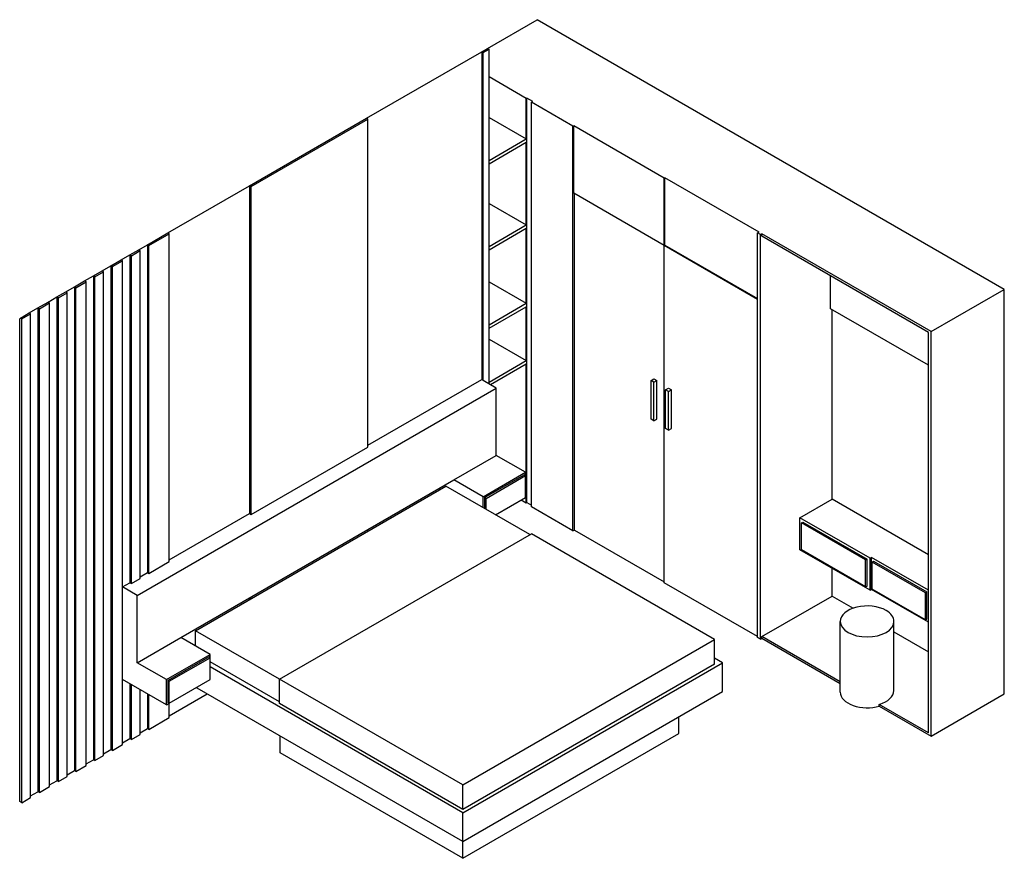
# Model space of a CAD drawing. Units: centimetres. Extents: x 2482 to 32323, y -172 to 5164.
# Tile 1 of 1: x 26482 to 32323, y 189 to 5164. Entities that reach past the tile are written whole.
import ezdxf

# ---------------------------------------------------------------- set-up
doc = ezdxf.new("R2010")
doc.units = ezdxf.units.CM
doc.header["$MEASUREMENT"] = 0
doc.layers.add('A-FURN', color=8, linetype='Continuous', lineweight=25)

msp = doc.modelspace()

# ---------------------------------------------------------------- linework, layer by layer
at = {"layer": 'A-FURN'}
for p, q in [((29257.4, 4994.3), (29551.8, 5164.3)), ((32323.1, 3564.3), (29551.8, 5164.3)), ((28538.6, 4579.3), (29222.7, 4974.3)), ((29222.7, 4974.3), (29257.4, 4994.3)), ((29231.4, 4969.3), (29222.7, 4974.3)), ((29222.7, 4974.3), (29222.7, 3029.3)), ((29231.4, 4969.3), (29266, 4989.3)), ((29231.4, 3024.3), (29231.4, 4969.3)), ((29257.4, 4994.3), (29266, 4989.3)), ((29266, 3004.3), (29266, 4989.3)), ((29486.9, 4696.8), (29266, 4824.3)), ((29486.9, 4696.8), (29491.2, 4699.3)), ((29486.9, 4456.8), (29486.9, 4696.8)), ((29525.8, 4679.3), (29491.2, 4699.3)), ((29491.2, 2299.3), (29491.2, 4699.3)), ((29517.2, 4674.3), (29525.8, 4679.3)), ((29764, 4531.8), (29517.2, 4674.3)), ((29517.2, 2274.3), (29517.2, 4674.3)), ((27845.7, 4179.3), (28538.6, 4579.3)), ((27854.4, 4174.3), (28547.2, 4574.3)), ((28547.2, 4574.3), (28538.6, 4579.3)), ((28547.2, 2629.3), (28547.2, 4574.3)), ((29266, 4584.3), (29486.9, 4456.8)), ((29764, 4531.8), (29768.3, 4534.3)), ((29764, 2131.8), (29764, 4531.8)), ((30305.3, 4224.3), (29768.3, 4534.3)), ((29768.3, 4134.3), (29768.3, 4534.3)), ((29266, 4329.3), (29486.9, 4456.8)), ((29266, 4309.3), (29486.9, 4436.8)), ((29486.9, 3946.8), (29486.9, 4436.8)), ((30305.3, 4224.3), (30309.6, 4226.8)), ((30305.3, 3824.3), (30305.3, 4224.3)), ((30868.2, 3904.3), (30309.6, 4226.8)), ((30309.6, 3826.8), (30309.6, 4226.8)), ((27360.8, 3899.3), (27845.7, 4179.3)), ((27845.7, 4179.3), (27845.7, 2234.3)), ((27854.4, 4174.3), (27845.7, 4179.3)), ((27854.4, 2229.3), (27854.4, 4174.3)), ((30305.3, 3824.3), (29768.3, 4134.3)), ((29772.7, 2136.8), (29772.7, 4131.8)), ((29266, 4074.3), (29486.9, 3946.8)), ((29266, 3819.3), (29486.9, 3946.8)), ((29266, 3799.3), (29486.9, 3926.8)), ((29486.9, 3481.8), (29486.9, 3926.8)), ((27239.5, 3829.3), (27360.8, 3899.3)), ((27248.2, 3824.3), (27369.4, 3894.3)), ((27369.4, 3894.3), (27360.8, 3899.3)), ((27369.4, 1949.3), (27369.4, 3894.3)), ((30859.5, 3899.3), (30868.2, 3904.3)), ((30876.8, 3889.3), (30859.5, 3899.3)), ((30859.5, 1499.3), (30859.5, 3899.3)), ((30876.8, 3889.3), (30885.5, 3894.3)), ((30876.8, 1489.3), (30876.8, 3889.3)), ((31890.1, 3314.3), (30885.5, 3894.3)), ((30885.5, 3879.3), (30885.5, 3894.3)), ((31872.8, 3309.3), (30885.5, 3879.3)), ((27135.6, 3769.3), (27187.6, 3799.3)), ((27187.6, 3799.3), (27239.5, 3829.3)), ((27196.2, 3794.3), (27187.6, 3799.3)), ((27239.5, 3829.3), (27239.5, 1884.3)), ((27248.2, 3824.3), (27239.5, 3829.3)), ((27248.2, 1879.3), (27248.2, 3824.3)), ((30305.3, 3824.3), (30309.6, 3826.8)), ((30305.3, 1824.3), (30305.3, 3824.3)), ((30859.5, 3504.3), (30305.3, 3824.3)), ((30309.6, 3826.8), (30859.5, 3509.3)), ((27023, 3704.3), (27083.6, 3739.3)), ((27083.6, 3739.3), (27135.6, 3769.3)), ((27092.3, 3734.3), (27083.6, 3739.3)), ((27135.6, 3769.3), (27135.6, 1824.3)), ((27144.3, 3764.3), (27135.6, 3769.3)), ((27144.3, 3764.3), (27196.2, 3794.3)), ((27144.3, 1819.3), (27144.3, 3764.3)), ((27196.2, 1849.3), (27196.2, 3794.3)), ((26971.1, 3674.3), (27023, 3704.3)), ((27023, 3704.3), (27023, 834.3)), ((27031.7, 3699.3), (27023, 3704.3)), ((27031.7, 3699.3), (27092.3, 3734.3)), ((27031.7, 829.3), (27031.7, 3699.3)), ((27092.3, 864.3), (27092.3, 3734.3)), ((26867.1, 3614.3), (26919.1, 3644.3)), ((26919.1, 3644.3), (26971.1, 3674.3)), ((26919.1, 3644.3), (26919.1, 774.3)), ((26927.8, 3639.3), (26919.1, 3644.3)), ((26927.8, 3639.3), (26979.7, 3669.3)), ((26927.8, 769.3), (26927.8, 3639.3)), ((26979.7, 3669.3), (26971.1, 3674.3)), ((26979.7, 799.3), (26979.7, 3669.3)), ((31292.5, 3449.3), (31292.5, 3644.3)), ((26754.6, 3549.3), (26806.5, 3579.3)), ((26806.5, 3579.3), (26867.1, 3614.3)), ((26806.5, 3579.3), (26806.5, 709.3)), ((26815.2, 3574.3), (26806.5, 3579.3)), ((26815.2, 3574.3), (26875.8, 3609.3)), ((26815.2, 704.3), (26815.2, 3574.3)), ((26875.8, 3609.3), (26867.1, 3614.3)), ((26875.8, 739.3), (26875.8, 3609.3)), ((29266, 3609.3), (29486.9, 3481.8)), ((31890.1, 3314.3), (32323.1, 3564.3)), ((32323.1, 1164.3), (32323.1, 3564.3)), ((26650.6, 3489.3), (26702.6, 3519.3)), ((26702.6, 3519.3), (26754.6, 3549.3)), ((26702.6, 3519.3), (26702.6, 649.3)), ((26711.3, 3514.3), (26702.6, 3519.3)), ((26711.3, 3514.3), (26763.2, 3544.3)), ((26711.3, 644.3), (26711.3, 3514.3)), ((26763.2, 3544.3), (26754.6, 3549.3)), ((26763.2, 674.3), (26763.2, 3544.3)), ((26538, 3424.3), (26590, 3454.3)), ((26590, 3454.3), (26650.6, 3489.3)), ((26590, 3454.3), (26590, 584.3)), ((26598.7, 3449.3), (26590, 3454.3)), ((26598.7, 3449.3), (26659.3, 3484.3)), ((26598.7, 579.3), (26598.7, 3449.3)), ((26659.3, 3484.3), (26650.6, 3489.3)), ((26659.3, 614.3), (26659.3, 3484.3)), ((29266, 3354.3), (29486.9, 3481.8)), ((29266, 3334.3), (29486.9, 3461.8)), ((29486.9, 3141.8), (29486.9, 3461.8)), ((31872.8, 3114.3), (31292.5, 3449.3)), ((26481.8, 3389.3), (26486.1, 3394.3)), ((26481.8, 526.8), (26481.8, 3389.3)), ((26486.1, 3394.3), (26538, 3424.3)), ((26494.7, 3389.3), (26486.1, 3394.3)), ((26494.7, 3389.3), (26546.7, 3419.3)), ((26494.7, 519.3), (26494.7, 3389.3)), ((26546.7, 3419.3), (26538, 3424.3)), ((26546.7, 549.3), (26546.7, 3419.3)), ((31301.2, 2319.3), (31301.2, 3444.3)), ((31872.8, 934.3), (31872.8, 3309.3)), ((31890.1, 914.3), (31890.1, 3314.3)), ((29266, 3269.3), (29486.9, 3141.8)), ((29266, 3014.3), (29486.9, 3141.8)), ((29274.7, 2999.3), (29486.9, 3121.8)), ((29486.9, 2296.8), (29486.9, 3121.8)), ((27178.9, 1749.3), (29309.3, 2979.3)), ((28547.2, 2639.3), (29222.7, 3029.3)), ((29231.4, 3024.3), (29222.7, 3029.3)), ((29309.3, 2979.3), (29231.4, 3024.3)), ((29309.3, 2579.3), (29309.3, 2979.3)), ((30227.3, 3024.3), (30244.6, 3034.3)), ((30227.3, 2794.3), (30227.3, 3024.3)), ((30244.6, 3014.3), (30227.3, 3024.3)), ((30244.6, 3034.3), (30262, 3024.3)), ((30244.6, 3014.3), (30262, 3024.3)), ((30244.6, 2784.3), (30244.6, 3014.3)), ((30262, 2794.3), (30262, 3024.3)), ((30313.9, 2969.3), (30331.2, 2979.3)), ((30331.2, 2979.3), (30348.6, 2969.3)), ((30313.9, 2739.3), (30313.9, 2969.3)), ((30331.2, 2959.3), (30313.9, 2969.3)), ((30331.2, 2959.3), (30348.6, 2969.3)), ((30331.2, 2729.3), (30331.2, 2959.3)), ((30348.6, 2739.3), (30348.6, 2969.3)), ((30244.6, 2784.3), (30227.3, 2794.3)), ((30244.6, 2784.3), (30262, 2794.3)), ((30331.2, 2729.3), (30313.9, 2739.3)), ((30331.2, 2729.3), (30348.6, 2739.3)), ((27854.4, 2229.3), (28547.2, 2629.3)), ((29058.2, 2434.3), (29309.3, 2579.3)), ((29482.5, 2479.3), (29309.3, 2579.3)), ((29231.4, 2334.3), (29482.5, 2479.3)), ((29240, 2329.3), (29473.9, 2464.3)), ((29248.7, 2324.3), (29482.5, 2459.3)), ((29482.5, 2459.3), (29473.9, 2464.3)), ((29482.5, 2459.3), (29482.5, 2479.3)), ((29482.5, 2329.3), (29482.5, 2459.3)), ((27438.7, 1499.3), (29058.2, 2434.3)), ((27525.3, 1539.3), (29010.6, 2396.8)), ((29508.5, 2109.3), (29010.6, 2396.8)), ((29231.4, 2334.3), (29058.2, 2434.3)), ((28971.6, 2384.3), (28971.6, 2374.3)), ((29231.4, 2269.3), (29231.4, 2334.3)), ((29240, 2329.3), (29240, 2264.3)), ((29248.7, 2324.3), (29240, 2329.3)), ((29248.7, 2259.3), (29248.7, 2324.3)), ((29305, 2226.8), (29482.5, 2329.3)), ((29486.9, 2296.8), (29456.6, 2314.3)), ((29486.9, 2296.8), (29491.2, 2299.3)), ((29491.2, 2299.3), (29517.2, 2284.3)), ((31110.7, 2209.3), (31301.2, 2319.3)), ((31872.8, 1989.3), (31301.2, 2319.3)), ((27369.4, 1959.3), (27845.7, 2234.3)), ((27845.7, 2234.3), (27854.4, 2229.3)), ((29764, 2131.8), (29517.2, 2274.3)), ((31110.7, 2019.3), (31110.7, 2209.3)), ((31526.4, 1969.3), (31110.7, 2209.3)), ((31119.3, 2179.3), (31128, 2184.3)), ((31119.3, 2019.3), (31119.3, 2179.3)), ((31500.4, 1959.3), (31119.3, 2179.3)), ((31128, 2184.3), (31509, 1964.3)), ((28023.3, 1251.8), (29517.2, 2114.3)), ((28547.2, 2129.3), (28547.2, 2139.3)), ((30604, 1486.8), (29517.2, 2114.3)), ((29764, 2131.8), (29772.7, 2136.8)), ((29772.7, 2136.8), (30305.3, 1829.3)), ((31526.4, 1779.3), (31110.7, 2019.3)), ((31500.4, 1799.3), (31119.3, 2019.3)), ((27248.2, 1879.3), (27369.4, 1949.3)), ((31500.4, 1959.3), (31509, 1964.3)), ((31500.4, 1799.3), (31500.4, 1959.3)), ((31509, 1804.3), (31509, 1964.3)), ((31526.4, 1969.3), (31535, 1974.3)), ((31526.4, 1779.3), (31526.4, 1969.3)), ((31872.8, 1779.3), (31535, 1974.3)), ((31535, 1784.3), (31535, 1974.3)), ((31539.3, 1946.8), (31548, 1951.8)), ((31539.3, 1786.8), (31539.3, 1946.8)), ((31855.4, 1764.3), (31539.3, 1946.8)), ((31548, 1951.8), (31864.1, 1769.3)), ((27196.2, 1859.3), (27239.5, 1884.3)), ((27239.5, 1884.3), (27248.2, 1879.3)), ((31301.2, 1744.3), (31301.2, 1909.3)), ((27092.3, 1799.3), (27135.6, 1824.3)), ((27135.6, 1824.3), (27144.3, 1819.3)), ((27144.3, 1819.3), (27196.2, 1849.3)), ((30859.5, 1504.3), (30305.3, 1824.3)), ((27178.9, 1749.3), (27092.3, 1799.3)), ((31500.4, 1799.3), (31509, 1804.3)), ((31526.4, 1779.3), (31535, 1784.3)), ((31872.8, 1589.3), (31535, 1784.3)), ((31855.4, 1604.3), (31539.3, 1786.8)), ((31855.4, 1764.3), (31864.1, 1769.3)), ((31855.4, 1604.3), (31855.4, 1764.3)), ((31864.1, 1609.3), (31864.1, 1769.3)), ((27178.9, 1349.3), (27178.9, 1749.3)), ((27845.7, 1734.3), (27845.7, 1724.3)), ((27854.4, 1729.3), (27854.4, 1739.3)), ((30885.5, 1504.3), (31301.2, 1744.3)), ((31301.2, 1744.3), (31425.5, 1672.5)), ((31349.8, 1174.3), (31349.8, 1594.3)), ((31668.3, 1184.3), (31668.3, 1594.3)), ((31855.4, 1604.3), (31864.1, 1609.3)), ((28023.3, 1251.8), (27525.3, 1539.3)), ((27525.3, 1449.3), (27525.3, 1539.3)), ((31668.3, 1532.3), (31872.8, 1414.3)), ((27178.9, 1349.3), (27438.7, 1499.3)), ((27611.9, 1399.3), (27438.7, 1499.3)), ((29110.1, 624.3), (30604, 1486.8)), ((30604, 1341.8), (30604, 1486.8)), ((30876.8, 1489.3), (30859.5, 1499.3)), ((30876.8, 1489.3), (30885.5, 1494.3)), ((30885.5, 1494.3), (30885.5, 1504.3)), ((31349.8, 1236.2), (30885.5, 1504.3)), ((30885.5, 1494.3), (31349.8, 1226.2)), ((27352.1, 1249.3), (27178.9, 1349.3)), ((27352.1, 1249.3), (27611.9, 1399.3)), ((27360.8, 1244.3), (27603.3, 1384.3)), ((27369.4, 1239.3), (27611.9, 1379.3)), ((27611.9, 1379.3), (27603.3, 1384.3)), ((27611.9, 1379.3), (27611.9, 1399.3)), ((27611.9, 1249.3), (27611.9, 1379.3)), ((28023.3, 1116.8), (27611.9, 1354.3)), ((29110.1, 459.3), (30651.7, 1349.3)), ((30651.7, 1349.3), (30604, 1376.8)), ((30651.7, 1179.3), (30651.7, 1349.3)), ((29110.1, 459.3), (27611.9, 1324.3)), ((30604, 1341.8), (29110.1, 479.3)), ((27352.1, 1099.3), (27092.3, 1249.3)), ((27352.1, 1099.3), (27352.1, 1249.3)), ((27360.8, 1244.3), (27360.8, 1114.3)), ((27369.4, 1239.3), (27360.8, 1244.3)), ((27369.4, 1109.3), (27611.9, 1249.3)), ((27369.4, 1109.3), (27369.4, 1239.3)), ((29110.1, 624.3), (28023.3, 1251.8)), ((28023.3, 1106.8), (28023.3, 1251.8)), ((27135.6, 1224.3), (27135.6, 899.3)), ((27144.3, 894.3), (27144.3, 1219.3)), ((27196.2, 924.3), (27196.2, 1189.3)), ((27534, 1199.3), (27534, 1204.3)), ((29110.1, 289.3), (27534, 1199.3)), ((29110.1, 289.3), (30651.7, 1179.3)), ((27239.5, 1164.3), (27239.5, 959.3)), ((27248.2, 954.3), (27248.2, 1159.3)), ((27369.4, 1109.3), (27360.8, 1114.3)), ((27369.4, 1034.3), (27594.6, 1164.3)), ((31890.1, 914.3), (32323.1, 1164.3)), ((27352.1, 1099.3), (27369.4, 1109.3)), ((27369.4, 1024.3), (27369.4, 1109.3)), ((29110.1, 479.3), (28023.3, 1106.8)), ((31872.8, 934.3), (31581.5, 1102.4)), ((31581.5, 1092.4), (31581.5, 1102.4)), ((31581.5, 1092.4), (31890.1, 914.3)), ((27248.2, 954.3), (27369.4, 1024.3)), ((30391.9, 929.3), (30391.9, 1029.3)), ((27196.2, 934.3), (27239.5, 959.3)), ((27248.2, 954.3), (27239.5, 959.3)), ((27092.3, 874.3), (27135.6, 899.3)), ((27144.3, 894.3), (27135.6, 899.3)), ((27144.3, 894.3), (27196.2, 924.3)), ((28027.6, 814.3), (28027.6, 914.3)), ((29110.1, 189.3), (30391.9, 929.3)), ((26979.7, 809.3), (27023, 834.3)), ((27031.7, 829.3), (27023, 834.3)), ((27031.7, 829.3), (27092.3, 864.3)), ((26875.8, 749.3), (26919.1, 774.3)), ((26927.8, 769.3), (26919.1, 774.3)), ((26927.8, 769.3), (26979.7, 799.3)), ((29110.1, 189.3), (28027.6, 814.3)), ((26763.2, 684.3), (26806.5, 709.3)), ((26815.2, 704.3), (26806.5, 709.3)), ((26815.2, 704.3), (26875.8, 739.3)), ((26659.3, 624.3), (26702.6, 649.3)), ((26711.3, 644.3), (26702.6, 649.3)), ((26711.3, 644.3), (26763.2, 674.3)), ((26546.7, 559.3), (26590, 584.3)), ((26598.7, 579.3), (26590, 584.3)), ((26598.7, 579.3), (26659.3, 614.3)), ((29110.1, 479.3), (29110.1, 624.3)), ((26494.7, 519.3), (26481.8, 526.8)), ((26494.7, 519.3), (26546.7, 549.3)), ((29110.1, 289.3), (29110.1, 459.3)), ((29110.1, 189.3), (29110.1, 289.3))]:
    msp.add_line(p, q, dxfattribs=at)
for centre, start_param, end_param in [((31509, 1594.3), 0.785398, 3.141593), ((31509, 1594.3), 0, 0.785398), ((31509, 1594.3), 3.141593, 6.283185), ((31509, 1174.3), 3.141593, 5.18502), ((31509, 1184.3), 5.18502, 6.283185)]:
    msp.add_ellipse(centre, major_axis=(159.2, 0), ratio=0.57735, start_param=start_param, end_param=end_param, dxfattribs=at)

doc.saveas('drawing.dxf')
